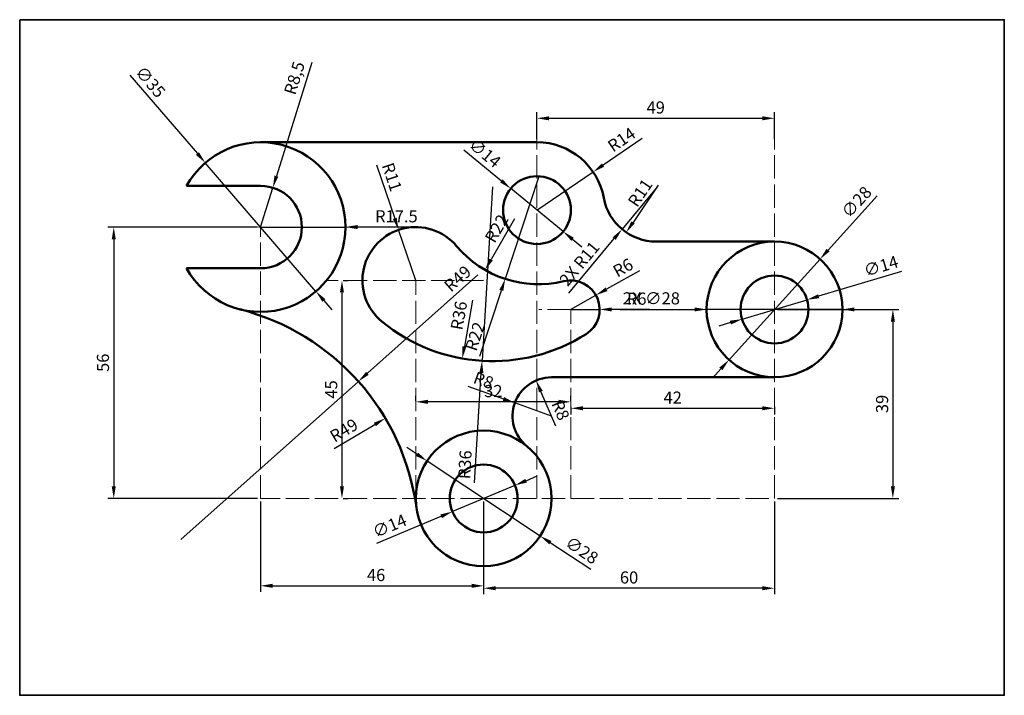
# Model space of a CAD drawing. Units: millimetres. Extents: x 76 to 280, y 64 to 203.
import ezdxf

# ---------------------------------------------------------------- set-up
doc = ezdxf.new("R2010")
doc.units = ezdxf.units.MM
doc.header["$LTSCALE"] = 0.4
doc.linetypes.add('ACAD_ISO02W100', pattern=[15, 12, -3])
for name, color, linetype, lineweight in [('M-CONS', 8, 'ACAD_ISO02W100', 18), ('M-DIMS', 2, 'Continuous', 25), ('M-OUTL', 7, 'Continuous', 50), ('M-TTLB', 7, 'Continuous', 35)]:
    doc.layers.add(name, color=color, linetype=linetype, lineweight=lineweight)
doc.styles.get("Standard").update_dxf_attribs({"font": 'arial.ttf'})
doc.dimstyles.new('ISO-25', dxfattribs={"dimtxt": 2.5, "dimasz": 2.5, "dimexe": 1.25, "dimexo": 0.625, "dimtad": 1, "dimtxsty": 'Standard', "dimcen": 2.5, "dimadec": 0, "dimazin": 0, "dimtfac": 1, "dimtmove": 0, "dimatfit": 3, "dimfxl": 1, "dimarcsym": 0})

# ---------------------------------------------------------------- blocks, each defined once
blk = doc.blocks.new('*D1')
at = {"layer": 'Defpoints', "color": 0, "ltscale": 0.4, "transparency": 16777216}
for p in [(190.15, 123.89), (232.15, 123.89), (232.15, 123)]:
    blk.add_point(p, dxfattribs=at)
at = {"layer": 'M-DIMS', "color": 0, "lineweight": -2, "ltscale": 0.4, "transparency": 16777216}
for p, q in [((190.15, 123.27), (190.15, 121.75)), ((192.65, 123), (229.65, 123)), ((232.15, 123.27), (232.15, 121.75))]:
    blk.add_line(p, q, dxfattribs=at)
at = {"layer": 'M-DIMS', "color": 0, "ltscale": 0.4, "transparency": 16777216}
for points in [[(192.65, 123.42), (192.65, 122.59), (190.15, 123)], [(229.65, 123.42), (229.65, 122.59), (232.15, 123)]]:
    blk.add_solid(points, dxfattribs=at)
at = {"layer": 'M-DIMS', "color": 0, "ltscale": 0.4, "transparency": 16777216, "insert": (211.15, 124.88), "char_height": 2.5, "attachment_point": 5}
blk.add_mtext('42', dxfattribs=at)
blk = doc.blocks.new('*D2')
at = {"layer": 'Defpoints', "color": 0, "ltscale": 0.4, "transparency": 16777216}
for p in [(158.15, 124.33), (158.15, 123.89), (190.15, 123.89)]:
    blk.add_point(p, dxfattribs=at)
at = {"layer": 'M-DIMS', "color": 0, "lineweight": -2, "ltscale": 0.4, "transparency": 16777216}
for p, q in [((158.15, 124.52), (158.15, 125.58)), ((187.65, 124.33), (160.65, 124.33)), ((190.15, 124.52), (190.15, 125.58))]:
    blk.add_line(p, q, dxfattribs=at)
at = {"layer": 'M-DIMS', "color": 0, "ltscale": 0.4, "transparency": 16777216}
for points in [[(160.65, 124.75), (160.65, 123.91), (158.15, 124.33)], [(187.65, 124.75), (187.65, 123.91), (190.15, 124.33)]]:
    blk.add_solid(points, dxfattribs=at)
at = {"layer": 'M-DIMS', "color": 0, "ltscale": 0.4, "transparency": 16777216, "insert": (174.15, 126.23), "char_height": 2.5, "attachment_point": 5}
blk.add_mtext('32', dxfattribs=at)
blk = doc.blocks.new('*D3')
at = {"layer": 'Defpoints', "color": 0, "ltscale": 0.4, "transparency": 16777216}
for p in [(232.15, 182.83), (183.15, 177.89), (232.15, 177.89)]:
    blk.add_point(p, dxfattribs=at)
at = {"layer": 'M-DIMS', "color": 0, "lineweight": -2, "ltscale": 0.4, "transparency": 16777216}
for p, q in [((183.15, 178.52), (183.15, 184.08)), ((185.65, 182.83), (229.65, 182.83)), ((232.15, 178.52), (232.15, 184.08))]:
    blk.add_line(p, q, dxfattribs=at)
at = {"layer": 'M-DIMS', "color": 0, "ltscale": 0.4, "transparency": 16777216}
for points in [[(185.65, 183.24), (185.65, 182.41), (183.15, 182.83)], [(229.65, 183.24), (229.65, 182.41), (232.15, 182.83)]]:
    blk.add_solid(points, dxfattribs=at)
at = {"layer": 'M-DIMS', "color": 0, "ltscale": 0.4, "transparency": 16777216, "insert": (207.65, 184.73), "char_height": 2.5, "attachment_point": 5}
blk.add_mtext('49', dxfattribs=at)
blk = doc.blocks.new('*D4')
at = {"layer": 'Defpoints', "color": 0, "ltscale": 0.4, "transparency": 16777216}
for p in [(232.15, 143.39), (232.15, 104.39), (256.57, 104.39)]:
    blk.add_point(p, dxfattribs=at)
at = {"layer": 'M-DIMS', "color": 0, "lineweight": -2, "ltscale": 0.4, "transparency": 16777216}
for p, q in [((232.78, 143.39), (257.82, 143.39)), ((256.57, 140.89), (256.57, 106.89)), ((232.78, 104.39), (257.82, 104.39))]:
    blk.add_line(p, q, dxfattribs=at)
at = {"layer": 'M-DIMS', "color": 0, "ltscale": 0.4, "transparency": 16777216}
for points in [[(256.15, 140.89), (256.99, 140.89), (256.57, 143.39)], [(256.15, 106.89), (256.99, 106.89), (256.57, 104.39)]]:
    blk.add_solid(points, dxfattribs=at)
at = {"layer": 'M-DIMS', "color": 0, "ltscale": 0.4, "transparency": 16777216, "insert": (254.67, 123.89), "char_height": 2.5, "attachment_point": 5, "rotation": 90}
blk.add_mtext('39', dxfattribs=at)
blk = doc.blocks.new('*D5')
at = {"layer": 'Defpoints', "color": 0, "ltscale": 0.4, "transparency": 16777216}
for p in [(172.15, 104.39), (232.15, 104.39), (172.15, 85.87)]:
    blk.add_point(p, dxfattribs=at)
at = {"layer": 'M-DIMS', "color": 0, "lineweight": -2, "ltscale": 0.4, "transparency": 16777216}
for p, q in [((172.15, 103.77), (172.15, 84.62)), ((232.15, 103.77), (232.15, 84.62)), ((229.65, 85.87), (174.65, 85.87))]:
    blk.add_line(p, q, dxfattribs=at)
at = {"layer": 'M-DIMS', "color": 0, "ltscale": 0.4, "transparency": 16777216}
for points in [[(174.65, 86.29), (174.65, 85.45), (172.15, 85.87)], [(229.65, 86.29), (229.65, 85.45), (232.15, 85.87)]]:
    blk.add_solid(points, dxfattribs=at)
at = {"layer": 'M-DIMS', "color": 0, "ltscale": 0.4, "transparency": 16777216, "insert": (202.15, 87.77), "char_height": 2.5, "attachment_point": 5}
blk.add_mtext('60', dxfattribs=at)
blk = doc.blocks.new('*D6')
at = {"layer": 'Defpoints', "color": 0, "ltscale": 0.4, "transparency": 16777216}
for p in [(126.15, 104.39), (172.15, 104.39), (172.15, 86.37)]:
    blk.add_point(p, dxfattribs=at)
at = {"layer": 'M-DIMS', "color": 0, "lineweight": -2, "ltscale": 0.4, "transparency": 16777216}
for p, q in [((126.15, 103.77), (126.15, 85.12)), ((172.15, 103.77), (172.15, 85.12)), ((128.65, 86.37), (169.65, 86.37))]:
    blk.add_line(p, q, dxfattribs=at)
at = {"layer": 'M-DIMS', "color": 0, "ltscale": 0.4, "transparency": 16777216}
for points in [[(128.65, 86.79), (128.65, 85.95), (126.15, 86.37)], [(169.65, 86.79), (169.65, 85.95), (172.15, 86.37)]]:
    blk.add_solid(points, dxfattribs=at)
at = {"layer": 'M-DIMS', "color": 0, "ltscale": 0.4, "transparency": 16777216, "insert": (149.97, 88.27), "char_height": 2.5, "attachment_point": 5}
blk.add_mtext('46', dxfattribs=at)
blk = doc.blocks.new('*D7')
at = {"layer": 'Defpoints', "color": 0, "ltscale": 0.4, "transparency": 16777216}
for p in [(142.57, 149.39), (142.57, 104.39), (142.93, 104.39)]:
    blk.add_point(p, dxfattribs=at)
at = {"layer": 'M-DIMS', "color": 0, "lineweight": -2, "ltscale": 0.4, "transparency": 16777216}
for p, q in [((143.19, 149.39), (144.18, 149.39)), ((142.93, 146.89), (142.93, 106.89)), ((143.19, 104.39), (144.18, 104.39))]:
    blk.add_line(p, q, dxfattribs=at)
at = {"layer": 'M-DIMS', "color": 0, "ltscale": 0.4, "transparency": 16777216}
for points in [[(142.51, 146.89), (143.34, 146.89), (142.93, 149.39)], [(142.51, 106.89), (143.34, 106.89), (142.93, 104.39)]]:
    blk.add_solid(points, dxfattribs=at)
at = {"layer": 'M-DIMS', "color": 0, "ltscale": 0.4, "transparency": 16777216, "insert": (141.03, 126.89), "char_height": 2.5, "attachment_point": 5, "rotation": 90}
blk.add_mtext('45', dxfattribs=at)
blk = doc.blocks.new('*D8')
at = {"layer": 'Defpoints', "color": 0, "ltscale": 0.4, "transparency": 16777216}
for p in [(126.15, 160.39), (95.85, 104.39), (126.15, 104.39)]:
    blk.add_point(p, dxfattribs=at)
at = {"layer": 'M-DIMS', "color": 0, "lineweight": -2, "ltscale": 0.4, "transparency": 16777216}
for p, q in [((125.53, 160.39), (94.6, 160.39)), ((95.85, 157.89), (95.85, 106.89)), ((125.53, 104.39), (94.6, 104.39))]:
    blk.add_line(p, q, dxfattribs=at)
at = {"layer": 'M-DIMS', "color": 0, "ltscale": 0.4, "transparency": 16777216}
for points in [[(95.44, 157.89), (96.27, 157.89), (95.85, 160.39)], [(95.44, 106.89), (96.27, 106.89), (95.85, 104.39)]]:
    blk.add_solid(points, dxfattribs=at)
at = {"layer": 'M-DIMS', "color": 0, "ltscale": 0.4, "transparency": 16777216, "insert": (93.95, 132.39), "char_height": 2.5, "attachment_point": 5, "rotation": 90}
blk.add_mtext('56', dxfattribs=at)
blk = doc.blocks.new('*D9')
at = {"layer": 'Defpoints', "color": 0, "ltscale": 0.4, "transparency": 16777216}
for p in [(114.74, 173.66), (137.57, 147.12)]:
    blk.add_point(p, dxfattribs=at)
at = {"layer": 'M-DIMS', "color": 0, "lineweight": -2, "ltscale": 0.4, "transparency": 16777216}
for p, q in [((99.2, 191.71), (113.11, 175.55)), ((137.57, 147.12), (114.74, 173.66)), ((139.2, 145.23), (140.83, 143.33))]:
    blk.add_line(p, q, dxfattribs=at)
at = {"layer": 'M-DIMS', "color": 0, "ltscale": 0.4, "transparency": 16777216}
for points in [[(113.43, 175.82), (112.79, 175.28), (114.74, 173.66)], [(139.51, 145.5), (138.88, 144.96), (137.57, 147.12)]]:
    blk.add_solid(points, dxfattribs=at)
at = {"layer": 'M-DIMS', "color": 0, "ltscale": 0.4, "transparency": 16777216, "insert": (103.17, 190.13), "char_height": 2.5, "attachment_point": 5, "rotation": 310.7093}
blk.add_mtext('∅35', dxfattribs=at)
blk = doc.blocks.new('*D10')
at = {"layer": 'Defpoints', "color": 0, "ltscale": 0.4, "transparency": 16777216}
for p in [(128.67, 168.51), (126.15, 160.39)]:
    blk.add_point(p, dxfattribs=at)
at = {"layer": 'M-DIMS', "color": 0, "lineweight": -2, "ltscale": 0.4, "transparency": 16777216}
for p, q in [((136.68, 194.34), (129.41, 170.9)), ((126.15, 160.39), (128.67, 168.51))]:
    blk.add_line(p, q, dxfattribs=at)
at = {"layer": 'M-DIMS', "color": 0, "ltscale": 0.4, "transparency": 16777216}
blk.add_solid([(129.01, 171.02), (129.81, 170.77), (128.67, 168.51)], dxfattribs=at)
at = {"layer": 'M-DIMS', "color": 0, "ltscale": 0.4, "transparency": 16777216, "insert": (133.43, 191.04), "char_height": 2.5, "attachment_point": 5, "rotation": 72.7695}
blk.add_mtext('R8,5', dxfattribs=at)
blk = doc.blocks.new('*D11')
at = {"layer": 'Defpoints', "color": 0, "ltscale": 0.4, "transparency": 16777216}
for p in [(154.62, 159.81), (158.15, 149.39)]:
    blk.add_point(p, dxfattribs=at)
at = {"layer": 'M-DIMS', "color": 0, "lineweight": -2, "ltscale": 0.4, "transparency": 16777216}
for p, q in [((150.08, 173.2), (153.82, 162.17)), ((158.15, 149.39), (154.62, 159.81))]:
    blk.add_line(p, q, dxfattribs=at)
at = {"layer": 'M-DIMS', "color": 0, "ltscale": 0.4, "transparency": 16777216}
blk.add_solid([(154.21, 162.31), (153.42, 162.04), (154.62, 159.81)], dxfattribs=at)
at = {"layer": 'M-DIMS', "color": 0, "ltscale": 0.4, "transparency": 16777216, "insert": (152.94, 170.61), "char_height": 2.5, "attachment_point": 5, "rotation": 288.742}
blk.add_mtext('R11', dxfattribs=at)
blk = doc.blocks.new('*D12')
at = {"layer": 'Defpoints', "color": 0, "ltscale": 0.4, "transparency": 16777216}
for p in [(183.44, 170.59), (172.44, 151.54)]:
    blk.add_point(p, dxfattribs=at)
at = {"layer": 'M-DIMS', "color": 0, "lineweight": -2, "ltscale": 0.4, "transparency": 16777216}
blk.add_line((178.54, 162.1), (173.69, 153.71), dxfattribs=at)
at = {"layer": 'M-DIMS', "color": 0, "ltscale": 0.4, "transparency": 16777216}
blk.add_solid([(173.33, 153.91), (174.05, 153.5), (172.44, 151.54)], dxfattribs=at)
at = {"layer": 'M-DIMS', "color": 0, "ltscale": 0.4, "transparency": 16777216, "insert": (175.11, 159.93), "char_height": 2.5, "attachment_point": 5, "rotation": 59.9865}
blk.add_mtext('R22', dxfattribs=at)
blk = doc.blocks.new('*D13')
at = {"layer": 'Defpoints', "color": 0, "ltscale": 0.4, "transparency": 16777216}
for p in [(174.01, 168.72), (167.75, 133.27)]:
    blk.add_point(p, dxfattribs=at)
at = {"layer": 'M-DIMS', "color": 0, "lineweight": -2, "ltscale": 0.4, "transparency": 16777216}
blk.add_line((169.87, 145.3), (168.18, 135.73), dxfattribs=at)
at = {"layer": 'M-DIMS', "color": 0, "ltscale": 0.4, "transparency": 16777216}
blk.add_solid([(167.77, 135.8), (168.59, 135.66), (167.75, 133.27)], dxfattribs=at)
at = {"layer": 'M-DIMS', "color": 0, "ltscale": 0.4, "transparency": 16777216, "insert": (167.37, 142.08), "char_height": 2.5, "attachment_point": 5, "rotation": 79.9809}
blk.add_mtext('R36', dxfattribs=at)
blk = doc.blocks.new('*D14')
at = {"layer": 'Defpoints', "color": 0, "ltscale": 0.4, "transparency": 16777216}
for p in [(195.32, 146.33), (190.08, 143.39)]:
    blk.add_point(p, dxfattribs=at)
at = {"layer": 'M-DIMS', "color": 0, "lineweight": -2, "ltscale": 0.4, "transparency": 16777216}
for p, q in [((204.28, 151.36), (197.5, 147.55)), ((190.08, 143.39), (195.32, 146.33))]:
    blk.add_line(p, q, dxfattribs=at)
at = {"layer": 'M-DIMS', "color": 0, "ltscale": 0.4, "transparency": 16777216}
blk.add_solid([(197.29, 147.92), (197.7, 147.19), (195.32, 146.33)], dxfattribs=at)
at = {"layer": 'M-DIMS', "color": 0, "ltscale": 0.4, "transparency": 16777216, "insert": (201.05, 151.73), "char_height": 2.5, "attachment_point": 5, "rotation": 29.3201}
blk.add_mtext('R6', dxfattribs=at)
blk = doc.blocks.new('*D15')
at = {"layer": 'Defpoints', "color": 0, "ltscale": 0.4, "transparency": 16777216}
for p in [(182.97, 128.75), (186.12, 121.39)]:
    blk.add_point(p, dxfattribs=at)
at = {"layer": 'M-DIMS', "color": 0, "lineweight": -2, "ltscale": 0.4, "transparency": 16777216}
blk.add_line((187.02, 119.29), (183.96, 126.45), dxfattribs=at)
at = {"layer": 'M-DIMS', "color": 0, "ltscale": 0.4, "transparency": 16777216}
blk.add_solid([(184.34, 126.61), (183.57, 126.28), (182.97, 128.75)], dxfattribs=at)
at = {"layer": 'M-DIMS', "color": 0, "ltscale": 0.4, "transparency": 16777216, "insert": (187.73, 122.47), "char_height": 2.5, "attachment_point": 5, "rotation": 293.1627}
blk.add_mtext('R8', dxfattribs=at)
blk = doc.blocks.new('*D16')
at = {"layer": 'Defpoints', "color": 0, "ltscale": 0.4, "transparency": 16777216}
for p in [(151.87, 120.94), (109.72, 95.95)]:
    blk.add_point(p, dxfattribs=at)
at = {"layer": 'M-DIMS', "color": 0, "lineweight": -2, "ltscale": 0.4, "transparency": 16777216}
blk.add_line((141.35, 114.7), (149.72, 119.66), dxfattribs=at)
at = {"layer": 'M-DIMS', "color": 0, "ltscale": 0.4, "transparency": 16777216}
blk.add_solid([(149.51, 120.02), (149.93, 119.31), (151.87, 120.94)], dxfattribs=at)
at = {"layer": 'M-DIMS', "color": 0, "ltscale": 0.4, "transparency": 16777216, "insert": (143.49, 118.18), "char_height": 2.5, "attachment_point": 5, "rotation": 30.6591}
blk.add_mtext('R49', dxfattribs=at)
blk = doc.blocks.new('*D17')
at = {"layer": 'Defpoints', "color": 0, "ltscale": 0.4, "transparency": 16777216}
for p in [(207.75, 168.39), (201.56, 159.29)]:
    blk.add_point(p, dxfattribs=at)
at = {"layer": 'M-DIMS', "color": 0, "lineweight": -2, "ltscale": 0.4, "transparency": 16777216}
blk.add_line((208.16, 169), (202.97, 161.36), dxfattribs=at)
at = {"layer": 'M-DIMS', "color": 0, "ltscale": 0.4, "transparency": 16777216}
blk.add_solid([(202.62, 161.59), (203.31, 161.13), (201.56, 159.29)], dxfattribs=at)
at = {"layer": 'M-DIMS', "color": 0, "ltscale": 0.4, "transparency": 16777216, "insert": (204.71, 167.27), "char_height": 2.5, "attachment_point": 5, "rotation": 55.797}
blk.add_mtext('R11', dxfattribs=at)
blk = doc.blocks.new('*D18')
at = {"layer": 'Defpoints', "color": 0, "ltscale": 0.4, "transparency": 16777216}
for p in [(194.73, 171.77), (183.15, 163.89)]:
    blk.add_point(p, dxfattribs=at)
at = {"layer": 'M-DIMS', "color": 0, "lineweight": -2, "ltscale": 0.4, "transparency": 16777216}
for p, q in [((204.82, 178.64), (196.79, 173.17)), ((183.15, 163.89), (194.73, 171.77))]:
    blk.add_line(p, q, dxfattribs=at)
at = {"layer": 'M-DIMS', "color": 0, "ltscale": 0.4, "transparency": 16777216}
blk.add_solid([(196.56, 173.52), (197.03, 172.83), (194.73, 171.77)], dxfattribs=at)
at = {"layer": 'M-DIMS', "color": 0, "ltscale": 0.4, "transparency": 16777216, "insert": (200.79, 178.16), "char_height": 2.5, "attachment_point": 5, "rotation": 34.2385}
blk.add_mtext('R14', dxfattribs=at)
blk = doc.blocks.new('*D19')
at = {"layer": 'Defpoints', "color": 0, "ltscale": 0.4, "transparency": 16777216}
for p in [(177.74, 168.33), (188.57, 159.45)]:
    blk.add_point(p, dxfattribs=at)
at = {"layer": 'M-DIMS', "color": 0, "lineweight": -2, "ltscale": 0.4, "transparency": 16777216}
for p, q in [((168.05, 176.29), (175.81, 169.92)), ((188.57, 159.45), (177.74, 168.33)), ((190.5, 157.86), (192.43, 156.28))]:
    blk.add_line(p, q, dxfattribs=at)
at = {"layer": 'M-DIMS', "color": 0, "ltscale": 0.4, "transparency": 16777216}
for points in [[(176.08, 170.24), (175.55, 169.6), (177.74, 168.33)], [(190.76, 158.19), (190.23, 157.54), (188.57, 159.45)]]:
    blk.add_solid(points, dxfattribs=at)
at = {"layer": 'M-DIMS', "color": 0, "ltscale": 0.4, "transparency": 16777216, "insert": (172.21, 175.42), "char_height": 2.5, "attachment_point": 5, "rotation": 320.6231}
blk.add_mtext('∅14', dxfattribs=at)
blk = doc.blocks.new('*D20')
at = {"layer": 'Defpoints', "color": 0, "ltscale": 0.4, "transparency": 16777216}
for p in [(241.54, 153.78), (222.77, 133)]:
    blk.add_point(p, dxfattribs=at)
at = {"layer": 'M-DIMS', "color": 0, "lineweight": -2, "ltscale": 0.4, "transparency": 16777216}
for p, q in [((253.31, 166.83), (243.21, 155.64)), ((222.77, 133), (241.54, 153.78)), ((221.1, 131.14), (219.42, 129.29))]:
    blk.add_line(p, q, dxfattribs=at)
at = {"layer": 'M-DIMS', "color": 0, "ltscale": 0.4, "transparency": 16777216}
for points in [[(242.9, 155.92), (243.52, 155.36), (241.54, 153.78)], [(220.79, 131.42), (221.41, 130.86), (222.77, 133)]]:
    blk.add_solid(points, dxfattribs=at)
at = {"layer": 'M-DIMS', "color": 0, "ltscale": 0.4, "transparency": 16777216, "insert": (249.31, 165.34), "char_height": 2.5, "attachment_point": 5, "rotation": 47.9265}
blk.add_mtext('∅28', dxfattribs=at)
blk = doc.blocks.new('*D21')
at = {"layer": 'Defpoints', "color": 0, "ltscale": 0.4, "transparency": 16777216}
for p in [(238.86, 145.39), (225.45, 141.39)]:
    blk.add_point(p, dxfattribs=at)
at = {"layer": 'M-DIMS', "color": 0, "lineweight": -2, "ltscale": 0.4, "transparency": 16777216}
for p, q in [((258.38, 151.22), (241.26, 146.11)), ((225.45, 141.39), (238.86, 145.39)), ((223.05, 140.67), (220.66, 139.96))]:
    blk.add_line(p, q, dxfattribs=at)
at = {"layer": 'M-DIMS', "color": 0, "ltscale": 0.4, "transparency": 16777216}
for points in [[(241.14, 146.51), (241.38, 145.71), (238.86, 145.39)], [(222.93, 141.07), (223.17, 140.27), (225.45, 141.39)]]:
    blk.add_solid(points, dxfattribs=at)
at = {"layer": 'M-DIMS', "color": 0, "ltscale": 0.4, "transparency": 16777216, "insert": (254.2, 152.03), "char_height": 2.5, "attachment_point": 5, "rotation": 16.6163}
blk.add_mtext('∅14', dxfattribs=at)
blk = doc.blocks.new('*D22')
at = {"layer": 'Defpoints', "color": 0, "ltscale": 0.4, "transparency": 16777216}
for p in [(160.49, 112.13), (183.82, 96.65)]:
    blk.add_point(p, dxfattribs=at)
at = {"layer": 'M-DIMS', "color": 0, "lineweight": -2, "ltscale": 0.4, "transparency": 16777216}
for p, q in [((158.4, 113.51), (156.32, 114.89)), ((160.49, 112.13), (183.82, 96.65)), ((194.29, 89.72), (185.91, 95.27))]:
    blk.add_line(p, q, dxfattribs=at)
at = {"layer": 'M-DIMS', "color": 0, "ltscale": 0.4, "transparency": 16777216}
for points in [[(158.63, 113.85), (158.17, 113.16), (160.49, 112.13)], [(186.14, 95.62), (185.68, 94.93), (183.82, 96.65)]]:
    blk.add_solid(points, dxfattribs=at)
at = {"layer": 'M-DIMS', "color": 0, "ltscale": 0.4, "transparency": 16777216, "insert": (192.23, 93.45), "char_height": 2.5, "attachment_point": 5, "rotation": 326.4572}
blk.add_mtext('∅28', dxfattribs=at)
blk = doc.blocks.new('*D23')
at = {"layer": 'Defpoints', "color": 0, "ltscale": 0.4, "transparency": 16777216}
for p in [(178.61, 107.1), (165.7, 101.68)]:
    blk.add_point(p, dxfattribs=at)
at = {"layer": 'M-DIMS', "color": 0, "lineweight": -2, "ltscale": 0.4, "transparency": 16777216}
for p, q in [((180.92, 108.06), (183.22, 109.03)), ((178.61, 107.1), (165.7, 101.68)), ((150.15, 95.17), (163.39, 100.72))]:
    blk.add_line(p, q, dxfattribs=at)
at = {"layer": 'M-DIMS', "color": 0, "ltscale": 0.4, "transparency": 16777216}
for points in [[(180.75, 108.45), (181.08, 107.68), (178.61, 107.1)], [(163.23, 101.1), (163.55, 100.33), (165.7, 101.68)]]:
    blk.add_solid(points, dxfattribs=at)
at = {"layer": 'M-DIMS', "color": 0, "ltscale": 0.4, "transparency": 16777216, "insert": (152.87, 98.44), "char_height": 2.5, "attachment_point": 5, "rotation": 22.7459}
blk.add_mtext('∅14', dxfattribs=at)
blk = doc.blocks.new('MOUNTING-BOSS-28-BORE-14')
for radius in [14, 7]:
    blk.add_circle((0, 0), radius)
blk = doc.blocks.new('*D25')
at = {"layer": 'Defpoints', "color": 0, "ltscale": 0.4, "transparency": 16777216}
for p in [(146.31, 128.55), (109.72, 95.95)]:
    blk.add_point(p, dxfattribs=at)
at = {"layer": 'M-DIMS', "color": 0, "lineweight": -2, "ltscale": 0.4, "transparency": 16777216}
for p, q in [((170.96, 150.51), (148.18, 130.21)), ((109.72, 95.95), (146.31, 128.55))]:
    blk.add_line(p, q, dxfattribs=at)
at = {"layer": 'M-DIMS', "color": 0, "ltscale": 0.4, "transparency": 16777216}
blk.add_solid([(147.9, 130.52), (148.45, 129.9), (146.31, 128.55)], dxfattribs=at)
at = {"layer": 'M-DIMS', "color": 0, "ltscale": 0.4, "transparency": 16777216, "insert": (167, 149.52), "char_height": 2.5, "attachment_point": 5, "rotation": 41.6951}
blk.add_mtext('R49', dxfattribs=at)
blk = doc.blocks.new('*D26')
at = {"layer": 'Defpoints', "color": 0, "ltscale": 0.4, "transparency": 16777216}
for p in [(174.01, 168.72), (171.82, 132.79)]:
    blk.add_point(p, dxfattribs=at)
at = {"layer": 'M-DIMS', "color": 0, "lineweight": -2, "ltscale": 0.4, "transparency": 16777216}
for p, q in [((174.01, 168.72), (171.82, 132.79)), ((170.29, 107.62), (171.67, 130.29))]:
    blk.add_line(p, q, dxfattribs=at)
at = {"layer": 'M-DIMS', "color": 0, "ltscale": 0.4, "transparency": 16777216}
blk.add_solid([(171.26, 130.32), (172.09, 130.27), (171.82, 132.79)], dxfattribs=at)
at = {"layer": 'M-DIMS', "color": 0, "ltscale": 0.4, "transparency": 16777216, "insert": (168.61, 111.34), "char_height": 2.5, "attachment_point": 5, "rotation": 86.5203}
blk.add_mtext('R36', dxfattribs=at)
blk = doc.blocks.new('*D27')
at = {"layer": 'Defpoints', "color": 0, "ltscale": 0.4, "transparency": 16777216}
for p in [(183.44, 170.59), (176.59, 149.69)]:
    blk.add_point(p, dxfattribs=at)
at = {"layer": 'M-DIMS', "color": 0, "lineweight": -2, "ltscale": 0.4, "transparency": 16777216}
for p, q in [((183.44, 170.59), (176.59, 149.69)), ((171.36, 133.72), (175.81, 147.31))]:
    blk.add_line(p, q, dxfattribs=at)
at = {"layer": 'M-DIMS', "color": 0, "ltscale": 0.4, "transparency": 16777216}
blk.add_solid([(175.41, 147.44), (176.21, 147.18), (176.59, 149.69)], dxfattribs=at)
at = {"layer": 'M-DIMS', "color": 0, "ltscale": 0.4, "transparency": 16777216, "insert": (170.69, 137.73), "char_height": 2.5, "attachment_point": 5, "rotation": 71.848}
blk.add_mtext('R22', dxfattribs=at)
blk = doc.blocks.new('*D28')
at = {"layer": 'Defpoints', "color": 0, "ltscale": 0.4, "transparency": 16777216}
for p in [(126.15, 160.39), (143.65, 160.39)]:
    blk.add_point(p, dxfattribs=at)
at = {"layer": 'M-DIMS', "color": 0, "lineweight": -2, "ltscale": 0.4, "transparency": 16777216}
for p, q in [((126.15, 160.39), (143.65, 160.39)), ((159.23, 160.39), (146.15, 160.39))]:
    blk.add_line(p, q, dxfattribs=at)
at = {"layer": 'M-DIMS', "color": 0, "ltscale": 0.4, "transparency": 16777216}
blk.add_solid([(146.15, 160.81), (146.15, 159.97), (143.65, 160.39)], dxfattribs=at)
at = {"layer": 'M-DIMS', "color": 0, "ltscale": 0.4, "transparency": 16777216, "insert": (154.15, 162.29), "char_height": 2.5, "attachment_point": 5, "rotation": 359.9985}
blk.add_mtext('R17.5', dxfattribs=at)
blk = doc.blocks.new('*D29')
at = {"layer": 'Defpoints', "color": 0, "ltscale": 0.4, "transparency": 16777216}
for p in [(218.15, 143.39), (246.15, 143.39)]:
    blk.add_point(p, dxfattribs=at)
at = {"layer": 'M-DIMS', "color": 0, "lineweight": -2, "ltscale": 0.4, "transparency": 16777216}
for p, q in [((200.32, 143.39), (215.65, 143.39)), ((246.15, 143.39), (218.15, 143.39)), ((248.65, 143.39), (251.15, 143.39))]:
    blk.add_line(p, q, dxfattribs=at)
at = {"layer": 'M-DIMS', "color": 0, "ltscale": 0.4, "transparency": 16777216}
for points in [[(215.65, 143.81), (215.65, 142.97), (218.15, 143.39)], [(248.65, 143.81), (248.65, 142.97), (246.15, 143.39)]]:
    blk.add_solid(points, dxfattribs=at)
at = {"layer": 'M-DIMS', "color": 0, "ltscale": 0.4, "transparency": 16777216, "insert": (206.74, 145.36), "char_height": 2.5, "attachment_point": 5, "rotation": 0.0019}
blk.add_mtext('2X ∅28', dxfattribs=at)
blk = doc.blocks.new('*D30')
at = {"layer": 'Defpoints', "color": 0, "ltscale": 0.4, "transparency": 16777216}
for p in [(207.75, 168.39), (200.7, 159.94)]:
    blk.add_point(p, dxfattribs=at)
at = {"layer": 'M-DIMS', "color": 0, "lineweight": -2, "ltscale": 0.4, "transparency": 16777216}
for p, q in [((207.75, 168.39), (200.7, 159.94)), ((189.72, 146.76), (199.1, 158.02))]:
    blk.add_line(p, q, dxfattribs=at)
at = {"layer": 'M-DIMS', "color": 0, "ltscale": 0.4, "transparency": 16777216}
blk.add_solid([(198.78, 158.29), (199.42, 157.75), (200.7, 159.94)], dxfattribs=at)
at = {"layer": 'M-DIMS', "color": 0, "ltscale": 0.4, "transparency": 16777216, "insert": (192.16, 152.64), "char_height": 2.5, "attachment_point": 5, "rotation": 50.1839}
blk.add_mtext('2X R11', dxfattribs=at)
blk = doc.blocks.new('*D31')
at = {"layer": 'Defpoints', "color": 0, "ltscale": 0.4, "transparency": 16777216}
for p in [(178.59, 124.09), (186.12, 121.39)]:
    blk.add_point(p, dxfattribs=at)
at = {"layer": 'M-DIMS', "color": 0, "lineweight": -2, "ltscale": 0.4, "transparency": 16777216}
for p, q in [((168.9, 127.55), (176.23, 124.93)), ((186.12, 121.39), (178.59, 124.09))]:
    blk.add_line(p, q, dxfattribs=at)
at = {"layer": 'M-DIMS', "color": 0, "ltscale": 0.4, "transparency": 16777216}
blk.add_solid([(176.37, 125.32), (176.09, 124.54), (178.59, 124.09)], dxfattribs=at)
at = {"layer": 'M-DIMS', "color": 0, "ltscale": 0.4, "transparency": 16777216, "insert": (172.03, 128.45), "char_height": 2.5, "attachment_point": 5, "rotation": 340.3007}
blk.add_mtext('R8', dxfattribs=at)
blk = doc.blocks.new('*D32')
at = {"layer": 'Defpoints', "color": 0, "ltscale": 0.4, "transparency": 16777216}
for p in [(190.08, 143.39), (196.08, 143.39)]:
    blk.add_point(p, dxfattribs=at)
at = {"layer": 'M-DIMS', "color": 0, "lineweight": -2, "ltscale": 0.4, "transparency": 16777216}
for p, q in [((190.08, 143.39), (196.08, 143.39)), ((206.36, 143.39), (198.58, 143.39))]:
    blk.add_line(p, q, dxfattribs=at)
at = {"layer": 'M-DIMS', "color": 0, "ltscale": 0.4, "transparency": 16777216}
blk.add_solid([(198.58, 143.81), (198.58, 142.97), (196.08, 143.39)], dxfattribs=at)
at = {"layer": 'M-DIMS', "color": 0, "ltscale": 0.4, "transparency": 16777216, "insert": (203.72, 145.29), "char_height": 2.5, "attachment_point": 5, "rotation": 359.9956}
blk.add_mtext('R6', dxfattribs=at)

msp = doc.modelspace()

# ---------------------------------------------------------------- linework, layer by layer
at = {"layer": 'M-CONS', "transparency": 33554572}
for p, q in [((183.154, 104.39), (183.154, 178.875)), ((232.154, 104.39), (232.154, 178.875)), ((107.731, 160.39), (148.669, 160.39)), ((126.154, 104.39), (126.154, 160.39)), ((172.154, 149.39), (139.765, 149.39)), ((158.154, 104.39), (158.154, 149.39)), ((232.154, 143.39), (183.531, 143.39)), ((190.154, 104.39), (190.154, 143.39)), ((172.154, 104.39), (126.154, 104.39)), ((172.154, 104.39), (232.154, 104.39))]:
    msp.add_line(p, q, dxfattribs=at)
at = {"layer": 'M-OUTL', "ltscale": 0.4}
for p, q in [((126.154, 177.89), (183.154, 177.89)), ((232.154, 157.39), (207.746, 157.39))]:
    msp.add_line(p, q, dxfattribs=at)
at = {"layer": 'M-OUTL'}
for p, q in [((126.154, 168.89), (110.857, 168.89)), ((126.154, 151.89), (110.857, 151.89)), ((232.154, 129.39), (186.118, 129.39))]:
    msp.add_line(p, q, dxfattribs=at)
at = {"layer": 'M-OUTL', "ltscale": 0.4}
msp.add_circle((183.154, 163.89), 7, dxfattribs=at)
at = {"layer": 'M-OUTL'}
for centre, radius, start, end in [((126.154, 160.39), 17.5, 209.05928, 150.94072), ((126.154, 160.39), 8.5, 270, 90), ((158.154, 149.39), 11, 39.97486, 230.6398), ((183.443, 170.591), 22, 219.97486, 283.7214), ((190.085, 143.39), 6, 302.40171, 103.7214), ((174.009, 168.72), 36, 230.6398, 302.40171), ((186.118, 121.39), 8, 90, 230.59943)]:
    msp.add_arc(centre, radius, start, end, dxfattribs=at)
at = {"layer": 'M-OUTL', "ltscale": 0.4}
for centre, radius, start, end in [((183.154, 163.89), 14, 10.36976, 90), ((207.746, 168.39), 11, 190.36976, 270), ((109.722, 95.953), 49, 7.69692, 75.69381)]:
    msp.add_arc(centre, radius, start, end, dxfattribs=at)
at = {"layer": 'M-TTLB', "ltscale": 0.4}
msp.add_lwpolyline([(76.45, 203.176), (279.555, 203.176), (279.555, 63.777), (76.45, 63.777)], close=True, dxfattribs=at)

# ---------------------------------------------------------------- block references
at = {"layer": 'M-OUTL'}
for p in [(232.154, 143.39), (172.154, 104.39)]:
    msp.add_blockref('MOUNTING-BOSS-28-BORE-14', p, dxfattribs=at)

# ---------------------------------------------------------------- dimensions: what is measured, and where the dimension line sits
at = {"layer": 'M-DIMS', "ltscale": 0.4}
for p1, p2, picture, middle in [((137.568, 147.125), (114.74, 173.656), '*D9', (101.671, 188.846)), ((222.773, 132.998), (241.535, 153.782), '*D20', (250.778, 164.021)), ((225.446, 141.389), (238.862, 145.392), '*D21', (254.766, 150.138)), ((178.61, 107.097), (165.699, 101.684), '*D23', (153.629, 96.624))]:
    dim = msp.add_diameter_dim_2p(p1=p1, p2=p2, dimstyle='ISO-25', override={"dimclrd": 0, "dimclre": 0, "dimclrt": 0}, dxfattribs=at)
    dim.commit()
    dim.dimension.update_dxf_attribs({"geometry": picture, "text_midpoint": middle, "dimtype": 163})
for center, mpoint, override, picture, middle in [((126.154, 160.39), (128.672, 168.509), {"dimclrd": 0, "dimclre": 0, "dimclrt": 0}, '*D10', (135.465, 190.413)), ((158.154, 149.39), (154.62, 159.807), {"dimclrd": 0, "dimclre": 0, "dimclrt": 0}, '*D11', (151.159, 170.008)), ((207.746, 168.39), (201.562, 159.293), {"dimclrd": 0, "dimclre": 0, "dimclrt": 0}, '*D17', (206.268, 166.216)), ((174.009, 168.72), (167.746, 133.269), {"dimclrd": 0, "dimclre": 0, "dimclrt": 0}, '*D13', (169.244, 141.749)), ((174.009, 168.72), (171.824, 132.786), {"dimdec": 0, "dimlfac": 1, "dimrnd": 0, "dimzin": 0, "dimdsep": 46, "dimlunit": 2}, '*D26', (170.513, 111.226)), ((183.443, 170.591), (176.589, 149.686), {"dimdec": 0, "dimlfac": 1, "dimrnd": 0, "dimzin": 0, "dimdsep": 46, "dimlunit": 2}, '*D27', (172.477, 137.143)), ((183.443, 170.591), (172.438, 151.541), {"dimclrd": 0, "dimclre": 0, "dimclrt": 0}, '*D12', (176.74, 158.987)), ((126.154, 160.39), (143.654, 160.39), {"dimdec": 1, "dimlfac": 1, "dimrnd": 0, "dimzin": 0, "dimdsep": 46, "dimlunit": 2}, '*D28', (154.154, 160.39)), ((109.722, 95.953), (146.31, 128.546), {"dimdec": 0, "dimlfac": 1, "dimrnd": 0, "dimzin": 0, "dimdsep": 46, "dimlunit": 2}, '*D25', (168.263, 148.102)), ((186.118, 121.39), (182.972, 128.746), {"dimclrd": 0, "dimclre": 0, "dimclrt": 0}, '*D15', (185.978, 121.718)), ((109.722, 95.953), (151.872, 120.939), {"dimclrd": 0, "dimclre": 0, "dimclrt": 0}, '*D16', (144.462, 116.546))]:
    dim = msp.add_radius_dim(center=center, mpoint=mpoint, dimstyle='ISO-25', override=override, dxfattribs=at)
    dim.commit()
    dim.dimension.update_dxf_attribs({"geometry": picture, "text_midpoint": middle, "dimtype": 164})
for base, p1, p2, picture, middle in [((232.154, 182.825), (183.154, 177.89), (232.154, 177.89), '*D3', (207.654, 184.726)), ((158.154, 124.33), (190.154, 123.89), (158.154, 123.89), '*D2', (174.154, 126.232)), ((232.154, 123.003), (190.154, 123.89), (232.154, 123.89), '*D1', (211.154, 124.883)), ((172.154, 85.868), (232.154, 104.39), (172.154, 104.39), '*D5', (202.154, 87.77))]:
    dim = msp.add_linear_dim(base=base, p1=p1, p2=p2, dimstyle='ISO-25', override={"dimclrd": 0, "dimclre": 0, "dimclrt": 0}, dxfattribs=at)
    dim.commit()
    dim.dimension.update_dxf_attribs({"geometry": picture, "text_midpoint": middle})
for center, mpoint, override, picture, middle in [((183.154, 163.89), (194.728, 171.767), {"dimclrd": 0, "dimclre": 0, "dimclrt": 0}, '*D18', (200.785, 178.164)), ((190.085, 143.39), (195.316, 146.329), {"dimclrd": 0, "dimclre": 0, "dimclrt": 0}, '*D14', (201.046, 151.728)), ((190.085, 143.39), (196.085, 143.39), {"dimdec": 0, "dimlfac": 1, "dimrnd": 0, "dimzin": 0, "dimdsep": 46, "dimlunit": 2}, '*D32', (203.725, 145.291)), ((186.118, 121.39), (178.587, 124.087), {"dimdec": 0, "dimlfac": 1, "dimrnd": 0, "dimzin": 0, "dimdsep": 46, "dimlunit": 2}, '*D31', (172.032, 128.454))]:
    dim = msp.add_radius_dim(center=center, mpoint=mpoint, dimstyle='ISO-25', override=override, dxfattribs=at)
    dim.commit()
    dim.dimension.update_dxf_attribs({"geometry": picture, "text_midpoint": middle})
for p1, p2, picture, middle in [((188.565, 159.45), (177.743, 168.331), '*D19', (172.214, 175.419)), ((160.486, 112.126), (183.823, 96.655), '*D22', (192.228, 93.447))]:
    dim = msp.add_diameter_dim_2p(p1=p1, p2=p2, dimstyle='ISO-25', override={"dimclrd": 0, "dimclre": 0, "dimclrt": 0}, dxfattribs=at)
    dim.commit()
    dim.dimension.update_dxf_attribs({"geometry": picture, "text_midpoint": middle})
dim = msp.add_radius_dim(center=(207.746, 168.39), mpoint=(200.702, 159.941), text='2X <>', dimstyle='ISO-25', override={"dimdec": 0, "dimlfac": 1, "dimrnd": 0, "dimzin": 0, "dimdsep": 46, "dimlunit": 2}, dxfattribs=at)
dim.commit()
dim.dimension.update_dxf_attribs({"geometry": '*D30', "text_midpoint": (192.164, 152.637)})
for base, p1, p2, picture, middle in [((95.854, 104.39), (126.154, 160.39), (126.154, 104.39), '*D8', (93.953, 132.39)), ((142.927, 104.39), (142.565, 149.39), (142.565, 104.39), '*D7', (141.031, 126.89)), ((256.57, 104.39), (232.154, 143.39), (232.154, 104.39), '*D4', (254.668, 123.89))]:
    dim = msp.add_linear_dim(base=base, p1=p1, p2=p2, angle=90, dimstyle='ISO-25', override={"dimclrd": 0, "dimclre": 0, "dimclrt": 0}, dxfattribs=at)
    dim.commit()
    dim.dimension.update_dxf_attribs({"geometry": picture, "text_midpoint": middle})
dim = msp.add_diameter_dim_2p(p1=(246.154, 143.391), p2=(218.154, 143.39), text='2X <>', dimstyle='ISO-25', override={"dimdec": 0, "dimlfac": 1, "dimrnd": 0, "dimzin": 0, "dimdsep": 46, "dimlunit": 2}, dxfattribs=at)
dim.commit()
dim.dimension.update_dxf_attribs({"geometry": '*D29', "text_midpoint": (206.735, 143.39)})
dim = msp.add_linear_dim(base=(172.154, 86.369), p1=(126.154, 104.39), p2=(172.154, 104.39), dimstyle='ISO-25', override={"dimclrd": 0, "dimclre": 0, "dimclrt": 0}, dxfattribs=at)
dim.commit()
dim.dimension.update_dxf_attribs({"geometry": '*D6', "text_midpoint": (149.968, 86.369), "dimtype": 160})

doc.saveas('drawing.dxf')
